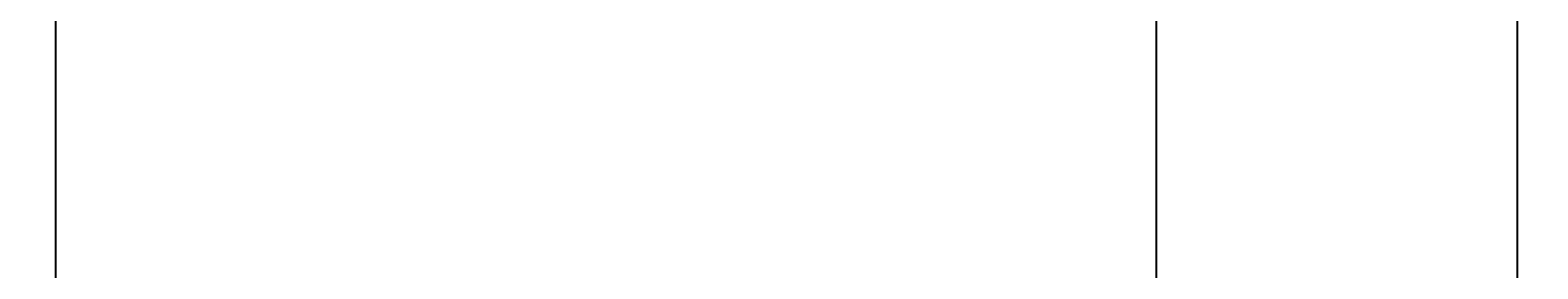
# Model space of a CAD drawing. Units: inches. Extents: x 35362 to 73946, y 43607 to 67532.
# Tile 80 of 134: x 50119 to 51337, y 47304 to 47497. Entities that reach past the tile are written whole.
import ezdxf

# ---------------------------------------------------------------- set-up
doc = ezdxf.new("R2010")
doc.units = ezdxf.units.IN
doc.header["$MEASUREMENT"] = 0
doc.layers.add('A-ANNO-DIMS', color=2, linetype='Continuous', lineweight=18)
doc.styles.get("Standard").update_dxf_attribs({"font": 'arial.ttf'})
doc.dimstyles.get("Standard").update_dxf_attribs({"dimtxt": 0.18, "dimasz": 0.18, "dimexe": 0.18, "dimexo": 0.0625, "dimgap": 0.09, "dimtad": 0, "dimtih": 1, "dimtoh": 1, "dimdec": 4, "dimzin": 0, "dimdsep": 46, "dimtxsty": 'Standard', "dimcen": 0.09, "dimadec": 0, "dimazin": 0, "dimtfac": 1, "dimtdec": 4, "dimtofl": 0, "dimtmove": 0, "dimatfit": 3, "dimfxl": 1, "dimtolj": 1, "dimtzin": 0, "dimarcsym": 0})

# ---------------------------------------------------------------- blocks, each defined once
blk = doc.blocks.new('*D11')
at = {"layer": 'A-ANNO-DIMS', "color": 0, "lineweight": -2, "transparency": 16777216}
for p, q in [((47978.7, 56028.8), (47978.7, 43606.7)), ((53109.8, 56028.8), (53109.8, 43606.7)), ((47978.8, 43606.9), (50543.9, 43606.9)), ((53109.6, 43606.9), (50544.6, 43606.9))]:
    blk.add_line(p, q, dxfattribs=at)
at = {"layer": 'A-ANNO-DIMS', "color": 0, "transparency": 16777216}
for points in [[(47978.8, 43606.9), (47978.8, 43606.8), (47978.7, 43606.9)], [(53109.6, 43606.9), (53109.6, 43606.8), (53109.8, 43606.9)]]:
    blk.add_solid(points, dxfattribs=at)
at = {"layer": 'Defpoints', "color": 0, "transparency": 16777216}
for p in [(47978.7, 56028.8), (53109.8, 56028.8), (53109.8, 43606.9)]:
    blk.add_point(p, dxfattribs=at)
at = {"layer": 'A-ANNO-DIMS', "color": 0, "transparency": 16777216, "insert": (50544.2, 43606.9), "char_height": 0.18, "attachment_point": 5}
blk.add_mtext('\\A1;5131', dxfattribs=at)
blk = doc.blocks.new('*D13')
at = {"layer": 'A-ANNO-DIMS', "color": 0, "lineweight": -2, "transparency": 16777216}
for p, q in [((48373.5, 51694), (48373.5, 43606.7)), ((51029, 51694), (51029, 43606.7)), ((48373.7, 43606.9), (49700.8, 43606.9)), ((51028.9, 43606.9), (49701.7, 43606.9))]:
    blk.add_line(p, q, dxfattribs=at)
at = {"layer": 'A-ANNO-DIMS', "color": 0, "transparency": 16777216}
for points in [[(48373.7, 43606.9), (48373.7, 43606.8), (48373.5, 43606.9)], [(51028.9, 43606.9), (51028.9, 43606.8), (51029, 43606.9)]]:
    blk.add_solid(points, dxfattribs=at)
at = {"layer": 'Defpoints', "color": 0, "transparency": 16777216}
for p in [(48373.5, 51694.1), (51029, 51694.1), (51029, 43606.9)]:
    blk.add_point(p, dxfattribs=at)
at = {"layer": 'A-ANNO-DIMS', "color": 0, "transparency": 16777216, "insert": (49701.3, 43606.9), "char_height": 0.18, "attachment_point": 5}
blk.add_mtext('\\A1;2655.6', dxfattribs=at)
blk = doc.blocks.new('*D17')
at = {"layer": 'A-ANNO-DIMS', "color": 0, "lineweight": -2, "transparency": 16777216}
for p, q in [((49923.3, 61293.2), (49923.3, 43606.7)), ((51913.9, 61293.2), (51913.9, 43606.7)), ((49923.5, 43606.9), (50918.2, 43606.9)), ((51913.8, 43606.9), (50919.1, 43606.9))]:
    blk.add_line(p, q, dxfattribs=at)
at = {"layer": 'A-ANNO-DIMS', "color": 0, "transparency": 16777216}
for points in [[(49923.5, 43606.9), (49923.5, 43606.8), (49923.3, 43606.9)], [(51913.8, 43606.9), (51913.8, 43606.8), (51913.9, 43606.9)]]:
    blk.add_solid(points, dxfattribs=at)
at = {"layer": 'Defpoints', "color": 0, "transparency": 16777216}
for p in [(49923.3, 61293.3), (51913.9, 61293.3), (51913.9, 43606.9)]:
    blk.add_point(p, dxfattribs=at)
at = {"layer": 'A-ANNO-DIMS', "color": 0, "transparency": 16777216, "insert": (50918.6, 43606.9), "char_height": 0.18, "attachment_point": 5}
blk.add_mtext('\\A1;1990.6', dxfattribs=at)
blk = doc.blocks.new('*D43')
at = {"layer": 'A-ANNO-DIMS', "color": 0, "lineweight": -2, "transparency": 16777216}
for p, q in [((62004.7, 47625.2), (35361.8, 47625.2)), ((35361.9, 47625), (35361.9, 47416.9)), ((35361.9, 47208.4), (35361.9, 47416.5)), ((62004.7, 47208.2), (35361.8, 47208.2))]:
    blk.add_line(p, q, dxfattribs=at)
at = {"layer": 'A-ANNO-DIMS', "color": 0, "transparency": 16777216}
for points in [[(35361.9, 47625), (35362, 47625), (35361.9, 47625.2)], [(35361.9, 47208.4), (35362, 47208.4), (35361.9, 47208.2)]]:
    blk.add_solid(points, dxfattribs=at)
at = {"layer": 'Defpoints', "color": 0, "transparency": 16777216}
for p in [(62004.7, 47625.2), (35361.9, 47208.2), (62004.7, 47208.2)]:
    blk.add_point(p, dxfattribs=at)
at = {"layer": 'A-ANNO-DIMS', "color": 0, "transparency": 16777216, "insert": (35361.9, 47416.7), "char_height": 0.18, "attachment_point": 5}
blk.add_mtext('\\A1;416.9', dxfattribs=at)
blk = doc.blocks.new('*D67')
at = {"layer": 'A-ANNO-DIMS', "color": 0, "lineweight": -2, "transparency": 16777216}
for p, q in [((56873.5, 53351.5), (35361.8, 53351.5)), ((35361.9, 53351.3), (35361.9, 49400.9)), ((35361.9, 45450.1), (35361.9, 49400.5)), ((53793.6, 45449.9), (35361.8, 45449.9))]:
    blk.add_line(p, q, dxfattribs=at)
at = {"layer": 'A-ANNO-DIMS', "color": 0, "transparency": 16777216}
for points in [[(35361.9, 53351.3), (35362, 53351.3), (35361.9, 53351.5)], [(35361.9, 45450.1), (35362, 45450.1), (35361.9, 45449.9)]]:
    blk.add_solid(points, dxfattribs=at)
at = {"layer": 'Defpoints', "color": 0, "transparency": 16777216}
for p in [(35361.9, 53351.5), (56873.6, 53351.5), (53793.6, 45449.9)]:
    blk.add_point(p, dxfattribs=at)
at = {"layer": 'A-ANNO-DIMS', "color": 0, "transparency": 16777216, "insert": (35361.9, 49400.7), "char_height": 0.18, "attachment_point": 5}
blk.add_mtext('\\A1;7901.6', dxfattribs=at)
blk = doc.blocks.new('*D107')
at = {"layer": 'A-ANNO-DIMS', "color": 0, "lineweight": -2, "transparency": 16777216}
for p, q in [((50139.6, 59850), (50139.6, 43606.7)), ((51320.8, 59850), (51320.8, 43606.7)), ((50139.7, 43606.9), (50729.7, 43606.9)), ((51320.6, 43606.9), (50730.6, 43606.9))]:
    blk.add_line(p, q, dxfattribs=at)
at = {"layer": 'A-ANNO-DIMS', "color": 0, "transparency": 16777216}
for points in [[(50139.7, 43606.9), (50139.7, 43606.8), (50139.6, 43606.9)], [(51320.6, 43606.9), (51320.6, 43606.8), (51320.8, 43606.9)]]:
    blk.add_solid(points, dxfattribs=at)
at = {"layer": 'Defpoints', "color": 0, "transparency": 16777216}
for p in [(50139.6, 59850.1), (51320.8, 59850.1), (51320.8, 43606.9)]:
    blk.add_point(p, dxfattribs=at)
at = {"layer": 'A-ANNO-DIMS', "color": 0, "transparency": 16777216, "insert": (50730.2, 43606.9), "char_height": 0.18, "attachment_point": 5}
blk.add_mtext('\\A1;1181.3', dxfattribs=at)

msp = doc.modelspace()

# ---------------------------------------------------------------- dimensions: what is measured, and where the dimension line sits
at = {"layer": 'A-ANNO-DIMS'}
for base, p1, p2, override, picture, middle in [((51913.931, 43606.859), (49923.307, 61293.286), (51913.931, 61293.286), {"dimdec": 1, "dimlfac": 1, "dimrnd": 0, "dimzin": 0, "dimdsep": 46, "dimlunit": 2}, '*D17', (50918.619, 43606.859)), ((51320.8133, 43606.859), (50139.5627, 59850.0769), (51320.8133, 59850.0769), {"dimdec": 1, "dimlfac": 1, "dimrnd": 0, "dimzin": 0, "dimdsep": 46, "dimlunit": 2}, '*D107', (50730.188, 43606.859)), ((53109.76, 43606.859), (47978.665, 56028.836), (53109.76, 56028.836), {"dimdec": 0, "dimlfac": 1, "dimrnd": 0, "dimzin": 0, "dimdsep": 46, "dimlunit": 2}, '*D11', (50544.212, 43606.859)), ((51029.043, 43606.859), (48373.492, 51694.087), (51029.043, 51694.087), {"dimdec": 1, "dimlfac": 1, "dimrnd": 0, "dimzin": 0, "dimdsep": 46, "dimlunit": 2}, '*D13', (49701.267, 43606.859))]:
    dim = msp.add_linear_dim(base=base, p1=p1, p2=p2, dimstyle='Standard', override=override, dxfattribs=at)
    dim.commit()
    dim.dimension.update_dxf_attribs({"geometry": picture, "text_midpoint": middle})
for base, p1, p2, picture, middle in [((35361.949, 53351.529), (53793.638, 45449.894), (56873.602, 53351.529), '*D67', (35361.949, 49400.712)), ((35361.949, 47208.25), (62004.728, 47625.181), (62004.728, 47208.25), '*D43', (35361.949, 47416.715))]:
    dim = msp.add_linear_dim(base=base, p1=p1, p2=p2, angle=90, dimstyle='Standard', override={"dimdec": 1, "dimlfac": 1, "dimrnd": 0, "dimzin": 0, "dimdsep": 46, "dimlunit": 2}, dxfattribs=at)
    dim.commit()
    dim.dimension.update_dxf_attribs({"geometry": picture, "text_midpoint": middle})

doc.saveas('drawing.dxf')
